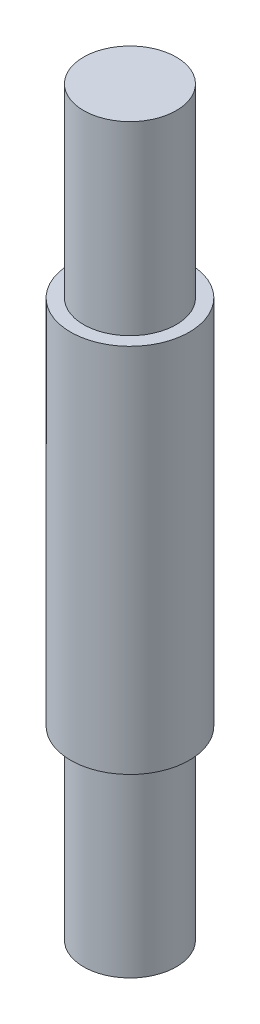
from build123d import *


with BuildPart() as part:
    # Pin Profile Sketch → Pin Body Revolve (revolve)
    with BuildSketch(Plane.XY, mode=Mode.PRIVATE) as pin_body_revolve_sk:
        Polygon((0, 0), (12.5, 0), (12.5, 50), (16, 50), (16, 150), (12.5, 150), (12.5, 200), (0, 200), align=None)
    revolve(pin_body_revolve_sk.sketch.rotate(Axis((0, 200, 0), (0, -1, 0)), 180), axis=Axis((0, 200, 0), (0, -1, 0)))


solid = part.part
